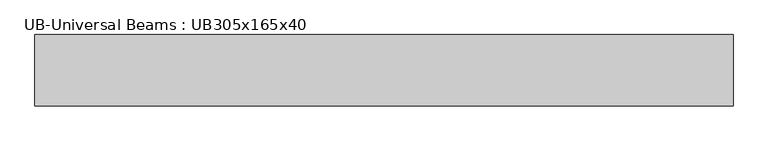
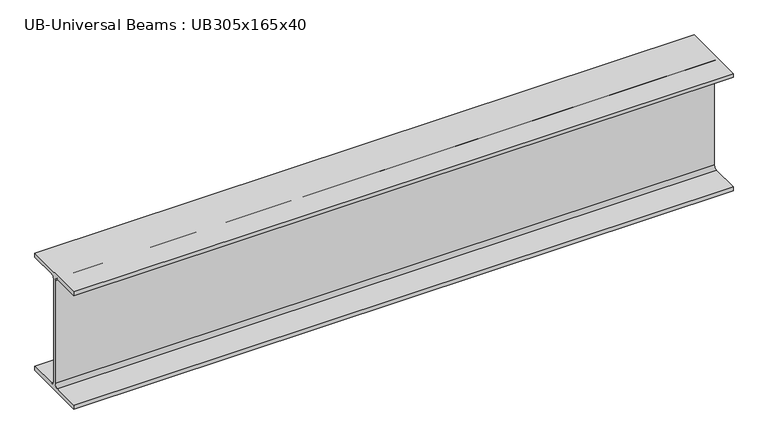
"""IFC4 building model written with IfcOpenShell, lengths in millimetres: beam geometry, UB-Universal Beams : UB305x165x40."""

from ifc_helpers import new_model, si_unit, point, frame, frame_2d, origin, place, context, project, spatial, polyline, circle_curve, trimmed, segment, composite_curve, outline, extrude, source, transform, mapped, element, save


def ub_universal_beams_ub305x165x40_862170f4(model_context):
    return source(origin(), model_context, "Body", "SweptSolid", [
        extrude(outline(composite_curve([segment(polyline([(82.5, -141.5), (82.5, -151.7), (-82.5, -151.7), (-82.5, -141.5), (-11.9, -141.5)]), True, "CONTINUOUS"), segment(trimmed(circle_curve(frame_2d((-11.9, -132.6)), 8.9), [point((-11.9, -141.5))], [point((-3.0, -132.6))], True, "CARTESIAN"), True, "CONTINUOUS"), segment(polyline([(-3.0, -132.6), (-3.0, 132.6)]), True, "CONTINUOUS"), segment(trimmed(circle_curve(frame_2d((-11.9, 132.6)), 8.9), [point((-3.0, 132.6))], [point((-11.9, 141.5))], True, "CARTESIAN"), True, "CONTINUOUS"), segment(polyline([(-11.9, 141.5), (-82.5, 141.5), (-82.5, 151.7), (82.5, 151.7), (82.5, 141.5), (11.9, 141.5)]), True, "CONTINUOUS"), segment(trimmed(circle_curve(frame_2d((11.9, 132.6)), 8.9), [point((11.9, 141.5))], [point((3.0, 132.6))], True, "CARTESIAN"), True, "CONTINUOUS"), segment(polyline([(3.0, 132.6), (3.0, -132.6)]), True, "CONTINUOUS"), segment(trimmed(circle_curve(frame_2d((11.9, -132.6)), 8.9), [point((3.0, -132.6))], [point((11.9, -141.5))], True, "CARTESIAN"), True, "CONTINUOUS"), segment(polyline([(11.9, -141.5), (82.5, -141.5)]), True, "CONTINUOUS")], self_intersect=False)), frame((-715.65, 0.0, 0.0), z_axis=(1.0, 0.0, 0.0), x_axis=(0.0, 1.0, 0.0)), (0.0, 0.0, 1.0), 1615.0),
    ])


if __name__ == "__main__":
    model = new_model("IFC4")
    model_context = context("Model", 3, world=origin())
    ifc_project = project(units=[si_unit("LENGTHUNIT", "METRE", prefix="MILLI")], contexts=[model_context])
    site = spatial("IfcSite", under=ifc_project)
    building = spatial("IfcBuilding", under=site)
    placement = place(None, origin())
    ub_universal_beams_ub305x165x40_shape = ub_universal_beams_ub305x165x40_862170f4(model_context)
    element("IfcBeam", 1, ObjectType="UB-Universal Beams : UB305x165x40", at=placement, inside=building, context=model_context, shape_type="MappedRepresentation", body=[
        mapped(ub_universal_beams_ub305x165x40_shape, transform((0.0, 0.0, 0.0), x_axis=(1.0, 0.0, 0.0), y_axis=(0.0, 1.0, 0.0), z_axis=(0.0, 0.0, 1.0))),
    ])
    save(model, "model.ifc")

# Revit data of these elements
# Type "UB-Universal Beams : UB305x165x40"
#   Section Name Key = "UB305X165X40"
#   Width = 16.5 cm
#   Web Thickness = 0.6 cm
#   Web Fillet = 0.89 cm
#   Warping Constant = 164000.0 cm⁶
#   Torsional Moment of Inertia = 14.70 cm⁴
#   Section Area = 51.3 cm²
#   Plastic Modulus weak axis = 142.0 cm³
#   Plastic Modulus strong axis = 623.0 cm³
#   Nominal Weight = 40.2999 kgf/m
#   Moment of Inertia weak axis = 764.00 cm⁴
#   Moment of Inertia strong axis = 8503.00 cm⁴
#   Height = 30.34 cm
#   Flange Thickness = 1.02 cm
#   Elastic Modulus weak axis = 92.6 cm³
#   Elastic Modulus strong axis = 560.0 cm³
#   Centroid Vertical = 15.17 cm
#   Centroid Horizontal = 8.25 cm
#   Bolt Spacing = 9.0 cm
#   Length [instance default] = 1500 mm
#   Structural Material [instance default] = Metal - Steel 43-275
#   Type Comments = ""
#   Assembly Code = ""
# Element 1 (IfcBeam, "UB-Universal Beams : UB305x165x40")
#   Materials on its faces: "Metal - Steel 43-275"
# Materials
#   "Metal - Steel 43-275": class "Metal", colour RGB 247 247 247, transparency 0, Cost = 0
